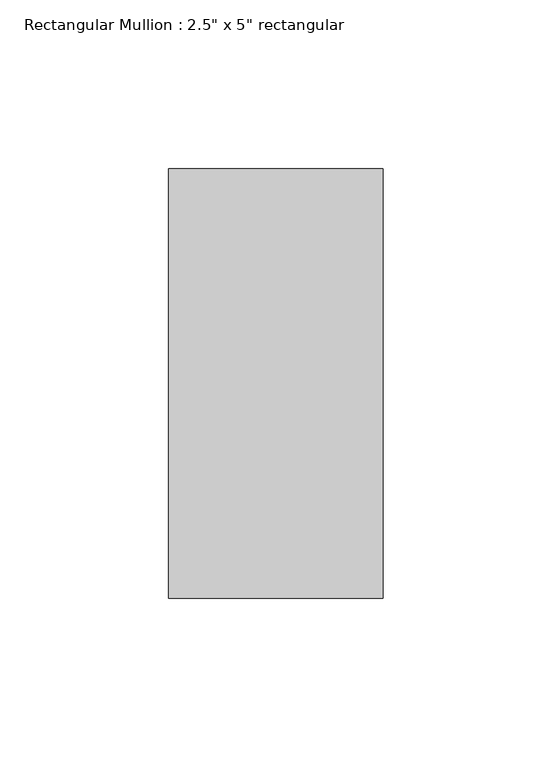
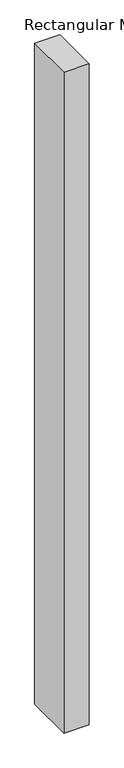
"""IFC4 building model written with IfcOpenShell, lengths in millimetres: member geometry."""

from ifc_helpers import new_model, si_unit, frame, origin, place, context, project, spatial, polyline, outline, extrude, source, transform, mapped, element, save


def member_6d95fc69(model_context):
    return source(origin(), model_context, "Body", "SweptSolid", [
        extrude(outline(polyline([(0.0, 63.5), (0.0, -63.5), (-63.5, -63.5), (-63.5, 63.5), (0.0, 63.5)])), frame((0.0, 0.0, -1755.4879691), z_axis=(0.0, 0.0, 1.0), x_axis=(1.0, 0.0, 0.0)), (0.0, 0.0, 1.0), 1755.4879691),
    ])


if __name__ == "__main__":
    model = new_model("IFC4")
    model_context = context("Model", 3, world=origin())
    ifc_project = project(units=[si_unit("LENGTHUNIT", "METRE", prefix="MILLI")], contexts=[model_context])
    site = spatial("IfcSite", under=ifc_project)
    building = spatial("IfcBuilding", under=site)
    placement = place(None, origin())
    member_shape = member_6d95fc69(model_context)
    element("IfcMember", 1, ObjectType="Rectangular Mullion : 2.5\" x 5\" rectangular", at=placement, inside=building, context=model_context, shape_type="MappedRepresentation", body=[
        mapped(member_shape, transform((0.0, 0.0, 0.0), x_axis=(1.0, 0.0, 0.0), y_axis=(0.0, 1.0, 0.0), z_axis=(0.0, 0.0, 1.0))),
    ])
    save(model, "model.ifc")

# Revit data of these elements
# Type "Rectangular Mullion : 2.5\" x 5\" rectangular"
#   built-in parameter 1007304 = 0.416667 (stored number, unit not read)
#   built-in parameter 1007301 = 0.104167 (stored number, unit not read)
#   built-in parameter 1007300 = 0.104167 (stored number, unit not read)
# Element 1 (IfcMember, "Rectangular Mullion : 2.5\" x 5\" rectangular")
#   Materials on its faces: "Aluminum"
# Materials
#   "Aluminum": class "Metal", colour RGB 247 247 247, transparency 0, Description = "Aluminum 6061", Cost = 0
